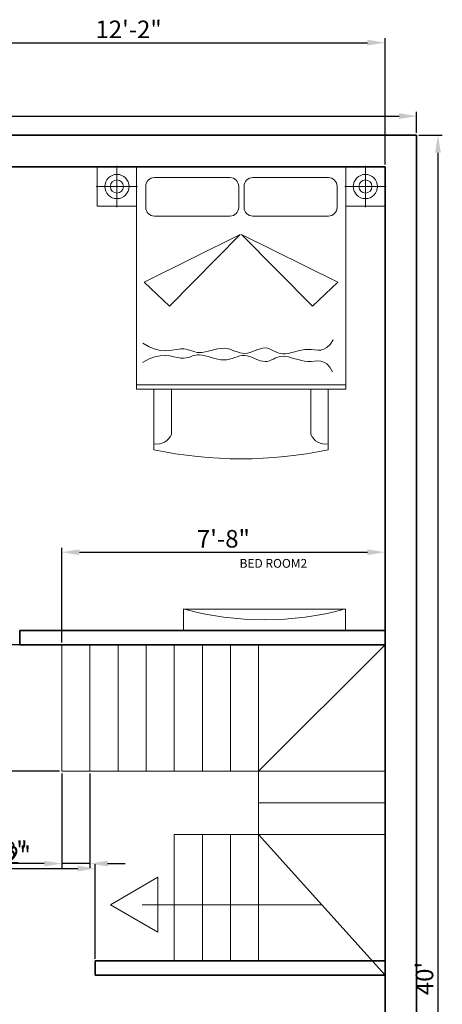
# Model space of a CAD drawing. Units: inches. Extents: x -24887 to 3061, y 1794 to 4919553.
# Tile 13 of 14: x 2941 to 3061, y 2190 to 2470. Entities that reach past the tile are written whole.
import ezdxf

# ---------------------------------------------------------------- set-up
doc = ezdxf.new("R2010")
doc.units = ezdxf.units.IN
for name, color, linetype, lineweight in [('A-ANNO-DIMS', 2, 'Continuous', 18), ('A-AREA-IDEN', 7, 'Continuous', 18), ('A-FLOR-STRS', 4, 'Continuous', 18), ('A-FURN', 8, 'Continuous', 18), ('TV', 210, 'Continuous', 18), ('wall', 7, 'Continuous', 35)]:
    doc.layers.add(name, color=color, linetype=linetype, lineweight=lineweight)
doc.styles.get("Standard").update_dxf_attribs({"font": 'arial.ttf'})
doc.dimstyles.new('ISO-25', dxfattribs={"dimtxt": 5, "dimasz": 5, "dimexe": 1.25, "dimexo": 0.625, "dimtad": 1, "dimdec": 1, "dimlunit": 3, "dimtxsty": 'Standard', "dimcen": 2.5, "dimadec": 0, "dimazin": 0, "dimtfac": 1, "dimtdec": 1, "dimtmove": 0, "dimatfit": 3, "dimfxl": 1, "dimarcsym": 0})

# ---------------------------------------------------------------- blocks, each defined once
blk = doc.blocks.new('A$C4F543DC7')
for p, q in [((0.013, 3.35, -0.169), (3.313, 3.35, -0.169)), ((0.463, 3.35, -0.169), (0.013, 3.35, -0.169)), ((0.013, 2.896, -0.169), (0.013, 3.35, -0.169)), ((0.013, 3.35, -0.169), (0.013, 2.896, -0.169)), ((0.238, 3.123, -0.439), (0.238, 3.361, -0.439)), ((0.463, 3.35, -0.169), (0.463, 0.8, -0.169)), ((2.863, 3.35, -0.169), (0.463, 3.35, -0.169)), ((0.463, 2.896, -0.169), (0.463, 3.35, -0.169)), ((2.863, 0.8, -0.169), (2.863, 3.35, -0.169)), ((2.863, 3.35, -0.169), (3.313, 3.35, -0.169)), ((2.863, 2.896, -0.169), (2.863, 3.35, -0.169)), ((3.089, 3.123, -0.439), (3.089, 3.361, -0.439)), ((3.313, 3.35, -0.169), (3.313, 2.896, -0.169)), ((3.313, 3.35, -0.169), (3.313, 2.896, -0.169)), ((1.535, 3.226, -0.169), (0.668, 3.226, -0.169)), ((2.664, 3.226, -0.169), (1.797, 3.226, -0.169)), ((0.238, 3.123, -0.439), (0, 3.123, -0.439)), ((0.238, 3.123, -0.439), (0.476, 3.123, -0.439)), ((0.238, 3.123, -0.439), (0.238, 2.885, -0.439)), ((0.568, 3.126, -0.169), (0.568, 2.884, -0.169)), ((1.635, 2.884, -0.169), (1.635, 3.126, -0.169)), ((1.697, 3.126, -0.169), (1.697, 2.884, -0.169)), ((2.764, 2.884, -0.169), (2.764, 3.126, -0.169)), ((3.089, 3.123, -0.439), (2.851, 3.123, -0.439)), ((3.089, 3.123, -0.439), (3.089, 2.885, -0.439)), ((3.089, 3.123, -0.439), (3.327, 3.123, -0.439)), ((0.463, 2.896, -0.169), (0.013, 2.896, -0.169)), ((0.013, 2.896, -0.169), (0.463, 2.896, -0.169)), ((0.463, 0.8, -0.169), (0.463, 2.896, -0.169)), ((2.863, 2.896, -0.169), (2.863, 0.8, -0.169)), ((3.313, 2.896, -0.169), (2.863, 2.896, -0.169)), ((3.313, 2.896, -0.169), (2.863, 2.896, -0.169)), ((0.668, 2.784, -0.169), (1.535, 2.784, -0.169)), ((1.797, 2.784, -0.169), (2.664, 2.784, -0.169)), ((1.653, 2.573, -0.169), (0.55, 2.025, -0.169)), ((0.841, 1.752, -0.169), (1.653, 2.573, -0.169)), ((2.481, 1.752, -0.169), (1.669, 2.573, -0.169)), ((1.669, 2.573, -0.169), (2.772, 2.025, -0.169)), ((0.55, 2.025, -0.169), (0.841, 1.752, -0.169)), ((2.772, 2.025, -0.169), (2.481, 1.752, -0.169)), ((2.683, 1.312, -0.169), (2.718, 1.364, -0.169)), ((0.537, 1.327, -0.169), (0.609, 1.284, -0.169)), ((0.609, 1.284, -0.169), (0.676, 1.257, -0.169)), ((0.676, 1.257, -0.169), (0.737, 1.243, -0.169)), ((0.737, 1.243, -0.169), (0.794, 1.239, -0.169)), ((0.794, 1.239, -0.169), (0.846, 1.242, -0.169)), ((0.846, 1.242, -0.169), (0.893, 1.249, -0.169)), ((0.893, 1.249, -0.169), (0.935, 1.256, -0.169)), ((0.935, 1.256, -0.169), (0.972, 1.261, -0.169)), ((0.972, 1.261, -0.169), (1.004, 1.262, -0.169)), ((1.004, 1.262, -0.169), (1.033, 1.258, -0.169)), ((1.033, 1.258, -0.169), (1.06, 1.251, -0.169)), ((1.06, 1.251, -0.169), (1.084, 1.242, -0.169)), ((1.084, 1.242, -0.169), (1.108, 1.234, -0.169)), ((1.285, 1.235, -0.169), (1.322, 1.244, -0.169)), ((1.322, 1.244, -0.169), (1.359, 1.253, -0.169)), ((1.359, 1.253, -0.169), (1.396, 1.261, -0.169)), ((1.396, 1.261, -0.169), (1.433, 1.266, -0.169)), ((1.433, 1.266, -0.169), (1.468, 1.268, -0.169)), ((1.468, 1.268, -0.169), (1.501, 1.264, -0.169)), ((1.501, 1.264, -0.169), (1.532, 1.257, -0.169)), ((1.532, 1.257, -0.169), (1.562, 1.247, -0.169)), ((1.562, 1.247, -0.169), (1.591, 1.237, -0.169)), ((1.826, 1.242, -0.169), (1.856, 1.253, -0.169)), ((1.856, 1.253, -0.169), (1.885, 1.263, -0.169)), ((1.885, 1.263, -0.169), (1.913, 1.27, -0.169)), ((1.913, 1.27, -0.169), (1.94, 1.272, -0.169)), ((1.94, 1.272, -0.169), (1.965, 1.269, -0.169)), ((1.965, 1.269, -0.169), (1.989, 1.262, -0.169)), ((1.989, 1.262, -0.169), (2.012, 1.251, -0.169)), ((2.012, 1.251, -0.169), (2.036, 1.239, -0.169)), ((2.317, 1.238, -0.169), (2.356, 1.246, -0.169)), ((2.356, 1.246, -0.169), (2.394, 1.253, -0.169)), ((2.394, 1.253, -0.169), (2.433, 1.255, -0.169)), ((2.433, 1.255, -0.169), (2.47, 1.253, -0.169)), ((2.47, 1.253, -0.169), (2.506, 1.249, -0.169)), ((2.506, 1.249, -0.169), (2.542, 1.246, -0.169)), ((2.542, 1.246, -0.169), (2.578, 1.248, -0.169)), ((2.578, 1.248, -0.169), (2.613, 1.257, -0.169)), ((2.613, 1.257, -0.169), (2.648, 1.277, -0.169)), ((2.648, 1.277, -0.169), (2.683, 1.312, -0.169)), ((0.533, 1.105, -0.169), (0.607, 1.146, -0.169)), ((0.607, 1.146, -0.169), (0.674, 1.171, -0.169)), ((0.674, 1.171, -0.169), (0.736, 1.183, -0.169)), ((0.736, 1.183, -0.169), (0.793, 1.185, -0.169)), ((0.793, 1.185, -0.169), (0.845, 1.18, -0.169)), ((0.845, 1.18, -0.169), (0.891, 1.172, -0.169)), ((0.891, 1.172, -0.169), (0.933, 1.163, -0.169)), ((0.933, 1.163, -0.169), (0.97, 1.156, -0.169)), ((0.97, 1.156, -0.169), (1.003, 1.155, -0.169)), ((1.003, 1.155, -0.169), (1.032, 1.158, -0.169)), ((1.032, 1.158, -0.169), (1.058, 1.164, -0.169)), ((1.058, 1.164, -0.169), (1.083, 1.172, -0.169)), ((1.083, 1.172, -0.169), (1.107, 1.18, -0.169)), ((1.107, 1.18, -0.169), (1.132, 1.187, -0.169)), ((1.108, 1.234, -0.169), (1.132, 1.226, -0.169)), ((1.132, 1.226, -0.169), (1.158, 1.22, -0.169)), ((1.132, 1.187, -0.169), (1.157, 1.192, -0.169)), ((1.157, 1.192, -0.169), (1.185, 1.193, -0.169)), ((1.158, 1.22, -0.169), (1.185, 1.218, -0.169)), ((1.185, 1.218, -0.169), (1.216, 1.22, -0.169)), ((1.185, 1.193, -0.169), (1.216, 1.19, -0.169)), ((1.216, 1.22, -0.169), (1.25, 1.226, -0.169)), ((1.216, 1.19, -0.169), (1.249, 1.183, -0.169)), ((1.249, 1.183, -0.169), (1.284, 1.173, -0.169)), ((1.25, 1.226, -0.169), (1.285, 1.235, -0.169)), ((1.284, 1.173, -0.169), (1.321, 1.163, -0.169)), ((1.321, 1.163, -0.169), (1.358, 1.152, -0.169)), ((1.358, 1.152, -0.169), (1.394, 1.143, -0.169)), ((1.394, 1.143, -0.169), (1.431, 1.137, -0.169)), ((1.431, 1.137, -0.169), (1.466, 1.135, -0.169)), ((1.466, 1.135, -0.169), (1.499, 1.137, -0.169)), ((1.499, 1.137, -0.169), (1.531, 1.143, -0.169)), ((1.531, 1.143, -0.169), (1.561, 1.152, -0.169)), ((1.561, 1.152, -0.169), (1.59, 1.162, -0.169)), ((1.59, 1.162, -0.169), (1.619, 1.172, -0.169)), ((1.591, 1.237, -0.169), (1.62, 1.226, -0.169)), ((1.619, 1.172, -0.169), (1.648, 1.18, -0.169)), ((1.62, 1.226, -0.169), (1.648, 1.217, -0.169)), ((1.648, 1.217, -0.169), (1.676, 1.211, -0.169)), ((1.648, 1.18, -0.169), (1.676, 1.185, -0.169)), ((1.676, 1.211, -0.169), (1.705, 1.209, -0.169)), ((1.676, 1.185, -0.169), (1.705, 1.186, -0.169)), ((1.705, 1.209, -0.169), (1.735, 1.212, -0.169)), ((1.705, 1.186, -0.169), (1.734, 1.182, -0.169)), ((1.734, 1.182, -0.169), (1.764, 1.173, -0.169)), ((1.735, 1.212, -0.169), (1.765, 1.22, -0.169)), ((1.764, 1.173, -0.169), (1.794, 1.162, -0.169)), ((1.765, 1.22, -0.169), (1.795, 1.23, -0.169)), ((1.794, 1.162, -0.169), (1.824, 1.149, -0.169)), ((1.795, 1.23, -0.169), (1.826, 1.242, -0.169)), ((1.824, 1.149, -0.169), (1.854, 1.137, -0.169)), ((1.854, 1.137, -0.169), (1.883, 1.126, -0.169)), ((1.987, 1.124, -0.169), (2.011, 1.134, -0.169)), ((2.011, 1.134, -0.169), (2.034, 1.145, -0.169)), ((2.034, 1.145, -0.169), (2.059, 1.157, -0.169)), ((2.036, 1.239, -0.169), (2.06, 1.227, -0.169)), ((2.059, 1.157, -0.169), (2.084, 1.167, -0.169)), ((2.06, 1.227, -0.169), (2.085, 1.216, -0.169)), ((2.084, 1.167, -0.169), (2.111, 1.174, -0.169)), ((2.085, 1.216, -0.169), (2.112, 1.208, -0.169)), ((2.111, 1.174, -0.169), (2.14, 1.177, -0.169)), ((2.112, 1.208, -0.169), (2.141, 1.204, -0.169)), ((2.14, 1.177, -0.169), (2.172, 1.175, -0.169)), ((2.141, 1.204, -0.169), (2.172, 1.205, -0.169)), ((2.172, 1.205, -0.169), (2.206, 1.21, -0.169)), ((2.172, 1.175, -0.169), (2.206, 1.169, -0.169)), ((2.206, 1.21, -0.169), (2.242, 1.218, -0.169)), ((2.206, 1.169, -0.169), (2.241, 1.16, -0.169)), ((2.241, 1.16, -0.169), (2.278, 1.149, -0.169)), ((2.242, 1.218, -0.169), (2.279, 1.228, -0.169)), ((2.278, 1.149, -0.169), (2.316, 1.138, -0.169)), ((2.279, 1.228, -0.169), (2.317, 1.238, -0.169)), ((2.316, 1.138, -0.169), (2.354, 1.128, -0.169)), ((1.883, 1.126, -0.169), (1.911, 1.119, -0.169)), ((1.911, 1.119, -0.169), (1.937, 1.115, -0.169)), ((1.937, 1.115, -0.169), (1.963, 1.118, -0.169)), ((1.963, 1.118, -0.169), (1.987, 1.124, -0.169)), ((2.354, 1.128, -0.169), (2.392, 1.121, -0.169)), ((2.392, 1.121, -0.169), (2.43, 1.117, -0.169)), ((2.43, 1.117, -0.169), (2.468, 1.118, -0.169)), ((2.468, 1.118, -0.169), (2.504, 1.121, -0.169)), ((2.504, 1.121, -0.169), (2.54, 1.123, -0.169)), ((2.54, 1.123, -0.169), (2.576, 1.12, -0.169)), ((2.576, 1.12, -0.169), (2.611, 1.109, -0.169)), ((2.611, 1.109, -0.169), (2.645, 1.088, -0.169)), ((2.645, 1.088, -0.169), (2.679, 1.052, -0.169)), ((2.679, 1.052, -0.169), (2.712, 0.999, -0.169)), ((0.463, 0.85, -0.169), (2.863, 0.85, -0.169)), ((0.463, 0.8, -0.169), (2.863, 0.8, -0.169)), ((0.663, 0.8, -0.169), (0.463, 0.8, -0.169)), ((0.663, 0.8, -0.169), (2.663, 0.8, -0.169)), ((0.663, 0.104, -0.169), (0.663, 0.8, -0.169)), ((0.663, 0.104, -0.169), (0.663, 0.8, -0.169)), ((0.863, 0.281, -0.169), (0.863, 0.8, -0.169)), ((2.463, 0.8, -0.169), (2.463, 0.281, -0.169)), ((2.863, 0.8, -0.169), (2.663, 0.8, -0.169)), ((2.663, 0.8, -0.169), (2.663, 0.104, -0.169)), ((2.663, 0.8, -0.169), (2.663, 0.104, -0.169))]:
    blk.add_line(p, q)
for centre, radius in [((0.238, 3.123, -0.439), 0.139), ((0.238, 3.123, -0.439), 0.075), ((3.089, 3.123, -0.439), 0.139), ((3.089, 3.123, -0.439), 0.075)]:
    blk.add_circle(centre, radius)
for centre, radius, start, end in [((0.668, 3.126, -0.169), 0.1, 90, 180), ((1.535, 3.126, -0.169), 0.1, 0, 90), ((1.797, 3.126, -0.169), 0.1, 90, 180), ((2.664, 3.126, -0.169), 0.1, 0, 90), ((0.668, 2.884, -0.169), 0.1, 180, 270), ((1.535, 2.884, -0.169), 0.1, 270, 0), ((1.797, 2.884, -0.169), 0.1, 180, 270), ((2.664, 2.884, -0.169), 0.1, 270, 0), ((0.699, 0.347, -0.169), 0.177, 258.2616, 338.032), ((2.627, 0.347, -0.169), 0.177, 201.968, 281.7384), ((1.663, 4.86, -0.169), 4.86, 258.1252, 281.8748), ((1.663, 4.86, -0.169), 4.86, 258.1252, 281.8748)]:
    blk.add_arc(centre, radius, start, end)
blk = doc.blocks.new('*D32')
at = {"layer": 'A-ANNO-DIMS', "color": 0, "lineweight": -2, "transparency": 16777216}
for p, q in [((2753.93, 2437.57), (2753.93, 2443.6)), ((3053.93, 2437.57), (3053.93, 2443.6)), ((2758.93, 2442.35), (3048.93, 2442.35))]:
    blk.add_line(p, q, dxfattribs=at)
at = {"layer": 'A-ANNO-DIMS', "color": 0, "transparency": 16777216}
for points in [[(2758.93, 2443.19), (2758.93, 2441.52), (2753.93, 2442.35)], [(3048.93, 2443.19), (3048.93, 2441.52), (3053.93, 2442.35)]]:
    blk.add_solid(points, dxfattribs=at)
at = {"layer": 'Defpoints', "color": 0, "transparency": 16777216}
for p in [(3053.93, 2442.35), (2753.93, 2436.94), (3053.93, 2436.94)]:
    blk.add_point(p, dxfattribs=at)
at = {"layer": 'A-ANNO-DIMS', "color": 0, "transparency": 16777216, "insert": (2903.93, 2445.53), "char_height": 5, "attachment_point": 5}
blk.add_mtext("25'", dxfattribs=at)
blk = doc.blocks.new('*D33')
at = {"layer": 'A-ANNO-DIMS', "color": 0, "lineweight": -2, "transparency": 16777216}
for p, q in [((3054.55, 2436.94), (3061.24, 2436.94)), ((3059.99, 2431.94), (3059.99, 1961.94)), ((3054.55, 1956.94), (3061.24, 1956.94))]:
    blk.add_line(p, q, dxfattribs=at)
at = {"layer": 'A-ANNO-DIMS', "color": 0, "transparency": 16777216}
for points in [[(3059.16, 2431.94), (3060.83, 2431.94), (3059.99, 2436.94)], [(3059.16, 1961.94), (3060.83, 1961.94), (3059.99, 1956.94)]]:
    blk.add_solid(points, dxfattribs=at)
at = {"layer": 'Defpoints', "color": 0, "transparency": 16777216}
for p in [(3053.93, 2436.94), (3053.93, 1956.94), (3059.99, 1956.94)]:
    blk.add_point(p, dxfattribs=at)
at = {"layer": 'A-ANNO-DIMS', "color": 0, "transparency": 16777216, "insert": (3056.82, 2196.94), "char_height": 5, "attachment_point": 5, "rotation": 90}
blk.add_mtext("40'", dxfattribs=at)
blk = doc.blocks.new('*D100')
at = {"layer": 'A-ANNO-DIMS', "color": 0, "lineweight": -2, "transparency": 16777216}
for p, q in [((2898.93, 2428.57), (2898.93, 2464.49)), ((2903.93, 2463.24), (3039.93, 2463.24)), ((3044.93, 2428.57), (3044.93, 2464.49))]:
    blk.add_line(p, q, dxfattribs=at)
at = {"layer": 'A-ANNO-DIMS', "color": 0, "transparency": 16777216}
for points in [[(2903.93, 2464.07), (2903.93, 2462.41), (2898.93, 2463.24)], [(3039.93, 2464.07), (3039.93, 2462.41), (3044.93, 2463.24)]]:
    blk.add_solid(points, dxfattribs=at)
at = {"layer": 'Defpoints', "color": 0, "transparency": 16777216}
for p in [(3044.93, 2463.24), (2898.93, 2427.94), (3044.93, 2427.94)]:
    blk.add_point(p, dxfattribs=at)
at = {"layer": 'A-ANNO-DIMS', "color": 0, "transparency": 16777216, "insert": (2971.93, 2466.38), "char_height": 5, "attachment_point": 5}
blk.add_mtext('12\'-2"', dxfattribs=at)
blk = doc.blocks.new('*D109')
at = {"layer": 'A-ANNO-DIMS', "color": 0, "lineweight": -2, "transparency": 16777216}
for p, q in [((2952.93, 2292.57), (2952.93, 2319.49)), ((2957.93, 2318.24), (3039.93, 2318.24)), ((3044.93, 2292.57), (3044.93, 2319.49))]:
    blk.add_line(p, q, dxfattribs=at)
at = {"layer": 'A-ANNO-DIMS', "color": 0, "transparency": 16777216}
for points in [[(2957.93, 2319.07), (2957.93, 2317.41), (2952.93, 2318.24)], [(3039.93, 2319.07), (3039.93, 2317.41), (3044.93, 2318.24)]]:
    blk.add_solid(points, dxfattribs=at)
at = {"layer": 'Defpoints', "color": 0, "transparency": 16777216}
for p in [(3044.93, 2318.24), (2952.93, 2291.94), (3044.93, 2291.94)]:
    blk.add_point(p, dxfattribs=at)
at = {"layer": 'A-ANNO-DIMS', "color": 0, "transparency": 16777216, "insert": (2998.93, 2321.42), "char_height": 5, "attachment_point": 5}
blk.add_mtext('7\'-8"', dxfattribs=at)
blk = doc.blocks.new('*D110')
at = {"layer": 'A-ANNO-DIMS', "color": 0, "lineweight": -2, "transparency": 16777216}
for p, q in [((2952.93, 2255.32), (2952.93, 2228.39)), ((2960.93, 2255.32), (2960.93, 2228.39)), ((2947.93, 2229.64), (2928.38, 2229.64)), ((2960.93, 2229.64), (2952.93, 2229.64)), ((2965.93, 2229.64), (2970.93, 2229.64))]:
    blk.add_line(p, q, dxfattribs=at)
at = {"layer": 'A-ANNO-DIMS', "color": 0, "transparency": 16777216}
for points in [[(2947.93, 2230.47), (2947.93, 2228.81), (2952.93, 2229.64)], [(2965.93, 2230.47), (2965.93, 2228.81), (2960.93, 2229.64)]]:
    blk.add_solid(points, dxfattribs=at)
at = {"layer": 'Defpoints', "color": 0, "transparency": 16777216}
for p in [(2952.93, 2255.94), (2960.93, 2255.94), (2952.93, 2229.64)]:
    blk.add_point(p, dxfattribs=at)
at = {"layer": 'A-ANNO-DIMS', "color": 0, "transparency": 16777216, "insert": (2935.66, 2232.82), "char_height": 5, "attachment_point": 5}
blk.add_mtext('0\'-8"', dxfattribs=at)
blk = doc.blocks.new('*D111')
at = {"layer": 'A-ANNO-DIMS', "color": 0, "lineweight": -2, "transparency": 16777216}
for p, q in [((2952.3, 2291.94), (2925.38, 2291.94)), ((2926.63, 2260.94), (2926.63, 2286.94)), ((2952.3, 2255.94), (2925.38, 2255.94))]:
    blk.add_line(p, q, dxfattribs=at)
at = {"layer": 'A-ANNO-DIMS', "color": 0, "transparency": 16777216}
for points in [[(2925.79, 2286.94), (2927.46, 2286.94), (2926.63, 2291.94)], [(2925.79, 2260.94), (2927.46, 2260.94), (2926.63, 2255.94)]]:
    blk.add_solid(points, dxfattribs=at)
at = {"layer": 'Defpoints', "color": 0, "transparency": 16777216}
for p in [(2926.63, 2291.94), (2952.93, 2291.94), (2952.93, 2255.94)]:
    blk.add_point(p, dxfattribs=at)
at = {"layer": 'A-ANNO-DIMS', "color": 0, "transparency": 16777216, "insert": (2923.45, 2273.94), "char_height": 5, "attachment_point": 5, "rotation": 90}
blk.add_mtext('3\'-0"', dxfattribs=at)
blk = doc.blocks.new('*D112')
at = {"layer": 'A-ANNO-DIMS', "color": 0, "lineweight": -2, "transparency": 16777216}
for p, q in [((2898.93, 2202.57), (2898.93, 2229.49)), ((2903.93, 2228.24), (2957.46, 2228.24)), ((2962.46, 2202.57), (2962.46, 2229.49))]:
    blk.add_line(p, q, dxfattribs=at)
at = {"layer": 'A-ANNO-DIMS', "color": 0, "transparency": 16777216}
for points in [[(2903.93, 2229.07), (2903.93, 2227.41), (2898.93, 2228.24)], [(2957.46, 2229.07), (2957.46, 2227.41), (2962.46, 2228.24)]]:
    blk.add_solid(points, dxfattribs=at)
at = {"layer": 'Defpoints', "color": 0, "transparency": 16777216}
for p in [(2962.46, 2228.24), (2898.93, 2201.94), (2962.46, 2201.94)]:
    blk.add_point(p, dxfattribs=at)
at = {"layer": 'A-ANNO-DIMS', "color": 0, "transparency": 16777216, "insert": (2930.69, 2231.45), "char_height": 5, "attachment_point": 5}
blk.add_mtext('5\'-3 1/2"', dxfattribs=at)

msp = doc.modelspace()

# ---------------------------------------------------------------- linework, layer by layer
at = {"layer": 'A-FLOR-STRS'}
for p, q in [((2952.93, 2291.94), (2952.93, 2255.94)), ((2952.93, 2291.94), (3008.93, 2291.94)), ((2960.93, 2291.94), (2960.93, 2255.94)), ((2968.93, 2291.94), (2968.93, 2255.94)), ((2976.93, 2291.94), (2976.93, 2255.94)), ((2984.93, 2291.94), (2984.93, 2255.94)), ((2992.93, 2291.94), (2992.93, 2255.94)), ((3000.93, 2291.94), (3000.93, 2255.94)), ((3044.93, 2291.94), (3008.93, 2291.94)), ((3008.93, 2291.94), (3008.93, 2255.94)), ((3008.93, 2255.94), (3044.93, 2291.94)), ((3044.93, 2255.94), (3044.93, 2291.94)), ((2952.93, 2255.94), (3008.93, 2255.94)), ((3008.93, 2255.94), (3044.93, 2255.94)), ((3008.93, 2255.94), (3008.93, 2237.94)), ((3044.93, 2255.94), (3044.93, 2237.94)), ((3008.93, 2246.94), (3044.93, 2246.94)), ((2984.93, 2237.94), (2984.93, 2201.94)), ((3008.93, 2237.94), (2984.93, 2237.94)), ((2992.93, 2237.94), (2992.93, 2201.94)), ((3000.93, 2237.94), (3000.93, 2201.94)), ((3044.93, 2237.94), (3008.93, 2237.94)), ((3008.93, 2237.94), (3008.93, 2201.94)), ((3008.93, 2237.94), (3044.93, 2237.94)), ((3008.93, 2237.94), (3044.93, 2197.94)), ((3044.93, 2201.94), (3044.93, 2237.94)), ((3026.93, 2217.94), (2975.78, 2217.94)), ((3008.93, 2201.94), (3044.93, 2201.94))]:
    msp.add_line(p, q, dxfattribs=at)
msp.add_lwpolyline([(2980.28, 2210.14), (2980.28, 2225.74), (2966.78, 2217.94)], close=True, dxfattribs=at)
at = {"layer": 'TV'}
msp.add_lwpolyline([(2987.53, 2295.94), (3033.72, 2295.94), (3033.72, 2302.09), (2987.53, 2302.09)], close=True, dxfattribs=at)
msp.add_arc((3010.62, 2387.3), 88.28, 254.8356, 285.1644, dxfattribs=at)
at = {"layer": 'wall'}
for p, q in [((3053.93, 2436.94), (2753.93, 2436.94)), ((3053.93, 1956.94), (3053.93, 2436.94)), ((3044.93, 2427.94), (2762.93, 2427.94)), ((3044.93, 1965.94), (3044.93, 2427.94)), ((3044.93, 2295.94), (2940.93, 2295.94)), ((2940.93, 2295.94), (2940.93, 2291.94)), ((3044.93, 2291.94), (2940.93, 2291.94)), ((3044.93, 2201.94), (2962.46, 2201.94)), ((2962.46, 2201.94), (2962.46, 2197.94)), ((3044.93, 2197.94), (2962.46, 2197.94))]:
    msp.add_line(p, q, dxfattribs=at)

# ---------------------------------------------------------------- block references
at = {"layer": 'A-FURN', "xscale": 24.81469674658305, "yscale": 24.81469674658305, "zscale": 24.81469674658305}
msp.add_blockref('A$C4F543DC7', (2962.7, 2344.81, 4.19), dxfattribs=at)

# ---------------------------------------------------------------- texts
at = {"layer": 'A-AREA-IDEN', "insert": (3003.53, 2316.33), "char_height": 2.5, "attachment_point": 1}
msp.add_mtext_dynamic_manual_height_columns('BED ROOM2', width=34.2323, gutter_width=12.5, heights=[0], dxfattribs=at)

# ---------------------------------------------------------------- dimensions: what is measured, and where the dimension line sits
at = {"layer": 'A-ANNO-DIMS'}
for base, p1, p2, override, picture, middle in [((3044.93, 2463.24), (2898.93, 2427.94), (3044.93, 2427.94), {"dimdec": 1, "dimlfac": 1, "dimrnd": 0, "dimzin": 1, "dimdsep": 46, "dimlunit": 4, "dimfrac": 2}, '*D100', (2971.93, 2466.38)), ((3053.93, 2442.35), (2753.93, 2436.94), (3053.93, 2436.94), {"dimclrd": 0, "dimclre": 0, "dimclrt": 0}, '*D32', (2903.93, 2445.53)), ((3044.93, 2318.24), (2952.93, 2291.94), (3044.93, 2291.94), {"dimdec": 1, "dimlfac": 1, "dimrnd": 0, "dimzin": 1, "dimdsep": 46, "dimlunit": 4, "dimfrac": 2}, '*D109', (2998.93, 2321.42)), ((2962.46, 2228.24), (2898.93, 2201.94), (2962.46, 2201.94), {"dimdec": 1, "dimlfac": 1, "dimrnd": 0, "dimzin": 1, "dimdsep": 46, "dimlunit": 4, "dimfrac": 2}, '*D112', (2930.69, 2231.45))]:
    dim = msp.add_linear_dim(base=base, p1=p1, p2=p2, dimstyle='ISO-25', override=override, dxfattribs=at)
    dim.commit()
    dim.dimension.update_dxf_attribs({"geometry": picture, "text_midpoint": middle})
for base, p1, p2, angle, override, picture, middle in [((3059.99, 1956.94), (3053.93, 2436.94), (3053.93, 1956.94), 90, {"dimclrd": 0, "dimclre": 0, "dimclrt": 0}, '*D33', (3056.82, 2196.94)), ((2926.63, 2291.94), (2952.93, 2255.94), (2952.93, 2291.94), 90, {"dimdec": 1, "dimlfac": 1, "dimrnd": 0, "dimzin": 1, "dimdsep": 46, "dimlunit": 4, "dimfrac": 2}, '*D111', (2923.45, 2273.94)), ((2952.93, 2229.64), (2960.93, 2255.94), (2952.93, 2255.94), 180, {"dimdec": 1, "dimlfac": 1, "dimrnd": 0, "dimzin": 1, "dimdsep": 46, "dimlunit": 4, "dimfrac": 2}, '*D110', (2935.66, 2232.82))]:
    dim = msp.add_linear_dim(base=base, p1=p1, p2=p2, angle=angle, dimstyle='ISO-25', override=override, dxfattribs=at)
    dim.commit()
    dim.dimension.update_dxf_attribs({"geometry": picture, "text_midpoint": middle})

doc.saveas('drawing.dxf')
